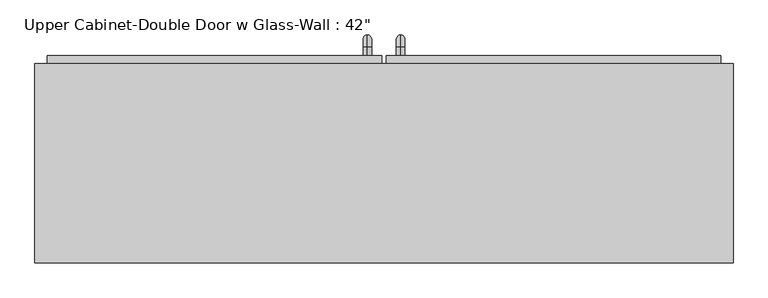
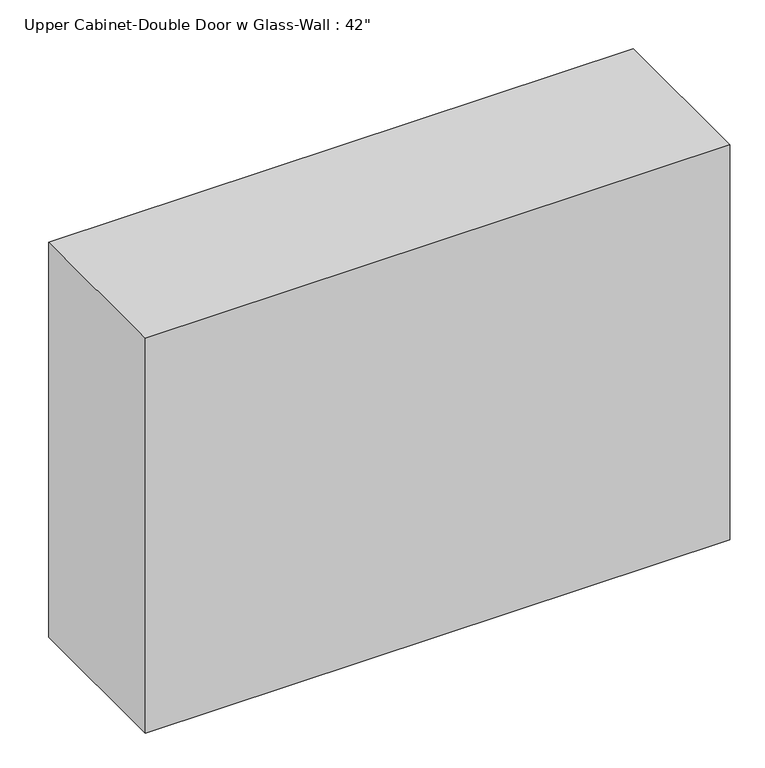
"""IFC4 building model written with IfcOpenShell, lengths in millimetres: furniture geometry."""

from ifc_helpers import new_model, si_unit, point, frame, origin, place, context, project, spatial, polyline, circle_curve, ellipse_curve, trimmed, outline, extrude, faceted_brep, source, transform, mapped, element, save
from ifc_brep_helpers import plane_surface, cylinder_surface, revolved_surface, advanced_brep


def furniture_92d3ea51(model_context):
    return source(origin(), model_context, "Body", "SolidModel", [
        extrude(outline(polyline([(2114.55, 32.9461628), (1390.65, 32.9461628), (1390.65, 544.1211628), (2114.55, 544.1211628), (2114.55, 32.9461628)]), holes=[polyline([(1422.4, 64.6961628), (2082.8, 64.6961628), (2082.8, 512.3711628), (1422.4, 512.3711628), (1422.4, 64.6961628)])]), frame((0.0, 342.9, 0.0), z_axis=(0.0, 1.0, 0.0), x_axis=(0.0, 0.0, 1.0)), (0.0, 0.0, 1.0), 31.75),
        extrude(outline(polyline([(1390.65, -484.5788372), (1390.65, 26.5961628), (2114.55, 26.5961628), (2114.55, -484.5788372), (1390.65, -484.5788372)]), holes=[polyline([(2082.8, -5.1538372), (1422.4, -5.1538372), (1422.4, -452.8288372), (2082.8, -452.8288372), (2082.8, -5.1538372)])]), frame((0.0, 342.9, 0.0), z_axis=(0.0, 1.0, 0.0), x_axis=(0.0, 0.0, 1.0)), (0.0, 0.0, 1.0), 31.75),
        extrude(outline(polyline([(64.6961628, 355.6), (512.3711628, 355.6), (512.3711628, 349.25), (64.6961628, 349.25), (64.6961628, 355.6)])), frame((0.0, 0.0, 1422.4), z_axis=(0.0, 0.0, 1.0), x_axis=(1.0, 0.0, 0.0)), (0.0, 0.0, 1.0), 660.4),
        extrude(outline(polyline([(-452.8288372, 355.6), (-5.1538372, 355.6), (-5.1538372, 349.25), (-452.8288372, 349.25), (-452.8288372, 355.6)])), frame((0.0, 0.0, 1422.4), z_axis=(0.0, 0.0, 1.0), x_axis=(1.0, 0.0, 0.0)), (0.0, 0.0, 1.0), 660.4),
        advanced_brep(
        [(4.3711628, 374.65, 1517.65), (4.3711628, 374.65, 1530.35), (4.3711628, 387.35, 1517.65), (4.3711628, 387.35, 1530.35), (4.3711628, 406.4, 1511.3), (4.3711628, 393.7, 1511.3), (4.3711628, 393.7, 1435.1), (4.3711628, 406.4, 1435.1), (4.3711628, 387.35, 1416.05), (4.3711628, 387.35, 1428.75), (4.3711628, 374.65, 1428.75), (4.3711628, 374.65, 1416.05)],
        [
            (0, 1, circle_curve(frame((4.3711628, 374.65, 1524.0), z_axis=(0.0, -1.0, 0.0), x_axis=(0.0, 0.0, 1.0)), 6.35)),
            (1, 0, circle_curve(frame((4.3711628, 374.65, 1524.0), z_axis=(0.0, -1.0, 0.0), x_axis=(0.0, 0.0, 1.0)), 6.35)),
            (0, 2),
            (2, 3, circle_curve(frame((4.3711628, 387.35, 1524.0), z_axis=(0.0, -1.0, 0.0), x_axis=(0.0, 0.0, 1.0)), 6.35)),
            (3, 1),
            (3, 2, circle_curve(frame((4.3711628, 387.35, 1524.0), z_axis=(0.0, -1.0, 0.0), x_axis=(0.0, 0.0, 1.0)), 6.35)),
            (4, 3, circle_curve(frame((4.3711628, 387.35, 1511.3), z_axis=(1.0, 0.0, 0.0), x_axis=(0.0, 0.0, 1.0)), 19.05)),
            (2, 5, circle_curve(frame((4.3711628, 387.35, 1511.3), z_axis=(-1.0, 0.0, 0.0), x_axis=(0.0, 0.0, 1.0)), 6.35)),
            (5, 4, circle_curve(frame((4.3711628, 400.05, 1511.3), z_axis=(0.0, 0.0, 1.0), x_axis=(0.0, 1.0, 0.0)), 6.35)),
            (4, 5, circle_curve(frame((4.3711628, 400.05, 1511.3), z_axis=(0.0, 0.0, 1.0), x_axis=(0.0, 1.0, 0.0)), 6.35)),
            (5, 6),
            (6, 7, circle_curve(frame((4.3711628, 400.05, 1435.1), z_axis=(0.0, 0.0, 1.0), x_axis=(0.0, 1.0, 0.0)), 6.35)),
            (7, 4),
            (7, 6, circle_curve(frame((4.3711628, 400.05, 1435.1), z_axis=(0.0, 0.0, 1.0), x_axis=(0.0, 1.0, 0.0)), 6.35)),
            (8, 7, circle_curve(frame((4.3711628, 387.35, 1435.1), z_axis=(1.0, 0.0, 0.0), x_axis=(0.0, 1.0, 0.0)), 19.05)),
            (6, 9, circle_curve(frame((4.3711628, 387.35, 1435.1), z_axis=(-1.0, 0.0, 0.0), x_axis=(0.0, 1.0, 0.0)), 6.35)),
            (9, 8, circle_curve(frame((4.3711628, 387.35, 1422.4), z_axis=(0.0, 1.0, 0.0), x_axis=(0.0, 0.0, -1.0)), 6.35)),
            (8, 9, circle_curve(frame((4.3711628, 387.35, 1422.4), z_axis=(0.0, 1.0, 0.0), x_axis=(0.0, 0.0, -1.0)), 6.35)),
            (10, 11, circle_curve(frame((4.3711628, 374.65, 1422.4), z_axis=(0.0, -1.0, 0.0), x_axis=(0.0, 0.0, -1.0)), 6.35)),
            (11, 10, circle_curve(frame((4.3711628, 374.65, 1422.4), z_axis=(0.0, -1.0, 0.0), x_axis=(0.0, 0.0, -1.0)), 6.35)),
            (9, 10),
            (11, 8),
        ],
        [
            plane_surface(frame((-1.9788372, 374.65, 1524.0), z_axis=(0.0, -1.0, 0.0), x_axis=(0.0, 0.0, 1.0))),
            cylinder_surface(frame((4.3711628, 374.65, 1524.0), z_axis=(0.0, -1.0, 0.0), x_axis=(0.0, 0.0, 1.0)), 6.35),
            revolved_surface(trimmed(ellipse_curve(frame((4.3711628, 387.35, 1524.0), z_axis=(0.0, -1.0, 0.0), x_axis=(0.0, 0.0, 1.0)), 6.35, 6.35), [point((4.3711628, 387.35, 1517.65))], [point((4.3711628, 387.35, 1530.35))], True, "CARTESIAN"), (4.3711628, 387.35, 1511.3), (-1.0, 0.0, 0.0)),
            revolved_surface(trimmed(ellipse_curve(frame((4.3711628, 387.35, 1524.0), z_axis=(0.0, -1.0, 0.0), x_axis=(0.0, 0.0, 1.0)), 6.35, 6.35), [point((4.3711628, 387.35, 1530.35))], [point((4.3711628, 387.35, 1517.65))], True, "CARTESIAN"), (4.3711628, 387.35, 1511.3), (-1.0, 0.0, 0.0)),
            cylinder_surface(frame((4.3711628, 400.05, 1511.3), z_axis=(0.0, 0.0, 1.0), x_axis=(0.0, 1.0, 0.0)), 6.35),
            revolved_surface(trimmed(ellipse_curve(frame((4.3711628, 400.05, 1435.1), z_axis=(0.0, 0.0, 1.0), x_axis=(0.0, 1.0, 0.0)), 6.35, 6.35), [point((4.3711628, 393.7, 1435.1))], [point((4.3711628, 406.4, 1435.1))], True, "CARTESIAN"), (4.3711628, 387.35, 1435.1), (-1.0, 0.0, 0.0)),
            revolved_surface(trimmed(ellipse_curve(frame((4.3711628, 400.05, 1435.1), z_axis=(0.0, 0.0, 1.0), x_axis=(0.0, 1.0, 0.0)), 6.35, 6.35), [point((4.3711628, 406.4, 1435.1))], [point((4.3711628, 393.7, 1435.1))], True, "CARTESIAN"), (4.3711628, 387.35, 1435.1), (-1.0, 0.0, 0.0)),
            plane_surface(frame((-1.9788372, 374.65, 1422.4), z_axis=(0.0, -1.0, 0.0), x_axis=(0.0, 0.0, -1.0))),
            cylinder_surface(frame((4.3711628, 387.35, 1422.4), z_axis=(0.0, 1.0, 0.0), x_axis=(0.0, 0.0, -1.0)), 6.35),
        ],
        [
            (0, [[1, 2]]),
            (1, [[-1, 3, 4, 5]]),
            (1, [[-2, -5, 6, -3]]),
            (2, [[7, -4, 8, 9]]),
            (3, [[-8, -6, -7, 10]]),
            (4, [[-9, 11, 12, 13]]),
            (4, [[-10, -13, 14, -11]]),
            (5, [[15, -12, 16, 17]]),
            (6, [[-16, -14, -15, 18]]),
            (7, [[19, 20]]),
            (8, [[-17, 21, -20, 22]]),
            (8, [[-18, -22, -19, -21]]),
        ],
    ),
        advanced_brep(
        [(55.1711628, 374.65, 1517.65), (55.1711628, 374.65, 1530.35), (55.1711628, 387.35, 1517.65), (55.1711628, 387.35, 1530.35), (55.1711628, 406.4, 1511.3), (55.1711628, 393.7, 1511.3), (55.1711628, 393.7, 1435.1), (55.1711628, 406.4, 1435.1), (55.1711628, 387.35, 1416.05), (55.1711628, 387.35, 1428.75), (55.1711628, 374.65, 1428.75), (55.1711628, 374.65, 1416.05)],
        [
            (0, 1, circle_curve(frame((55.1711628, 374.65, 1524.0), z_axis=(0.0, -1.0, 0.0), x_axis=(0.0, 0.0, -1.0)), 6.35)),
            (1, 0, circle_curve(frame((55.1711628, 374.65, 1524.0), z_axis=(0.0, -1.0, 0.0), x_axis=(0.0, 0.0, -1.0)), 6.35)),
            (0, 2),
            (2, 3, circle_curve(frame((55.1711628, 387.35, 1524.0), z_axis=(0.0, -1.0, 0.0), x_axis=(0.0, 0.0, -1.0)), 6.35)),
            (3, 1),
            (3, 2, circle_curve(frame((55.1711628, 387.35, 1524.0), z_axis=(0.0, -1.0, 0.0), x_axis=(0.0, 0.0, -1.0)), 6.35)),
            (4, 3, circle_curve(frame((55.1711628, 387.35, 1511.3), z_axis=(1.0, 0.0, 0.0), x_axis=(0.0, 0.0, 1.0)), 19.05)),
            (2, 5, circle_curve(frame((55.1711628, 387.35, 1511.3), z_axis=(-1.0, 0.0, 0.0), x_axis=(0.0, 0.0, 1.0)), 6.35)),
            (5, 4, circle_curve(frame((55.1711628, 400.05, 1511.3), z_axis=(0.0, 0.0, 1.0), x_axis=(0.0, -1.0, 0.0)), 6.35)),
            (4, 5, circle_curve(frame((55.1711628, 400.05, 1511.3), z_axis=(0.0, 0.0, 1.0), x_axis=(0.0, -1.0, 0.0)), 6.35)),
            (5, 6),
            (6, 7, circle_curve(frame((55.1711628, 400.05, 1435.1), z_axis=(0.0, 0.0, 1.0), x_axis=(0.0, -1.0, 0.0)), 6.35)),
            (7, 4),
            (7, 6, circle_curve(frame((55.1711628, 400.05, 1435.1), z_axis=(0.0, 0.0, 1.0), x_axis=(0.0, -1.0, 0.0)), 6.35)),
            (8, 7, circle_curve(frame((55.1711628, 387.35, 1435.1), z_axis=(1.0, 0.0, 0.0), x_axis=(0.0, 1.0, 0.0)), 19.05)),
            (6, 9, circle_curve(frame((55.1711628, 387.35, 1435.1), z_axis=(-1.0, 0.0, 0.0), x_axis=(0.0, 1.0, 0.0)), 6.35)),
            (9, 8, circle_curve(frame((55.1711628, 387.35, 1422.4), z_axis=(0.0, 1.0, 0.0), x_axis=(0.0, 0.0, 1.0)), 6.35)),
            (8, 9, circle_curve(frame((55.1711628, 387.35, 1422.4), z_axis=(0.0, 1.0, 0.0), x_axis=(0.0, 0.0, 1.0)), 6.35)),
            (10, 11, circle_curve(frame((55.1711628, 374.65, 1422.4), z_axis=(0.0, -1.0, 0.0), x_axis=(0.0, 0.0, 1.0)), 6.35)),
            (11, 10, circle_curve(frame((55.1711628, 374.65, 1422.4), z_axis=(0.0, -1.0, 0.0), x_axis=(0.0, 0.0, 1.0)), 6.35)),
            (9, 10),
            (11, 8),
        ],
        [
            plane_surface(frame((48.8211628, 374.65, 1524.0), z_axis=(0.0, -1.0, 0.0), x_axis=(0.0, 0.0, 1.0))),
            cylinder_surface(frame((55.1711628, 374.65, 1524.0), z_axis=(0.0, -1.0, 0.0), x_axis=(0.0, 0.0, -1.0)), 6.35),
            revolved_surface(trimmed(ellipse_curve(frame((55.1711628, 387.35, 1524.0), z_axis=(0.0, -1.0, 0.0), x_axis=(0.0, 0.0, -1.0)), 6.35, 6.35), [point((55.1711628, 387.35, 1517.65))], [point((55.1711628, 387.35, 1530.35))], True, "CARTESIAN"), (55.1711628, 387.35, 1511.3), (-1.0, 0.0, 0.0)),
            revolved_surface(trimmed(ellipse_curve(frame((55.1711628, 387.35, 1524.0), z_axis=(0.0, -1.0, 0.0), x_axis=(0.0, 0.0, -1.0)), 6.35, 6.35), [point((55.1711628, 387.35, 1530.35))], [point((55.1711628, 387.35, 1517.65))], True, "CARTESIAN"), (55.1711628, 387.35, 1511.3), (-1.0, 0.0, 0.0)),
            cylinder_surface(frame((55.1711628, 400.05, 1511.3), z_axis=(0.0, 0.0, 1.0), x_axis=(0.0, -1.0, 0.0)), 6.35),
            revolved_surface(trimmed(ellipse_curve(frame((55.1711628, 400.05, 1435.1), z_axis=(0.0, 0.0, 1.0), x_axis=(0.0, -1.0, 0.0)), 6.35, 6.35), [point((55.1711628, 393.7, 1435.1))], [point((55.1711628, 406.4, 1435.1))], True, "CARTESIAN"), (55.1711628, 387.35, 1435.1), (-1.0, 0.0, 0.0)),
            revolved_surface(trimmed(ellipse_curve(frame((55.1711628, 400.05, 1435.1), z_axis=(0.0, 0.0, 1.0), x_axis=(0.0, -1.0, 0.0)), 6.35, 6.35), [point((55.1711628, 406.4, 1435.1))], [point((55.1711628, 393.7, 1435.1))], True, "CARTESIAN"), (55.1711628, 387.35, 1435.1), (-1.0, 0.0, 0.0)),
            plane_surface(frame((48.8211628, 374.65, 1422.4), z_axis=(0.0, -1.0, 0.0), x_axis=(0.0, 0.0, -1.0))),
            cylinder_surface(frame((55.1711628, 387.35, 1422.4), z_axis=(0.0, 1.0, 0.0), x_axis=(0.0, 0.0, 1.0)), 6.35),
        ],
        [
            (0, [[1, 2]]),
            (1, [[-1, 3, 4, 5]]),
            (1, [[-2, -5, 6, -3]]),
            (2, [[7, -4, 8, 9]]),
            (3, [[-8, -6, -7, 10]]),
            (4, [[-9, 11, 12, 13]]),
            (4, [[-10, -13, 14, -11]]),
            (5, [[15, -12, 16, 17]]),
            (6, [[-16, -14, -15, 18]]),
            (7, [[19, 20]]),
            (8, [[-17, 21, -20, 22]]),
            (8, [[-18, -22, -19, -21]]),
        ],
    ),
        faceted_brep([(-503.6288372, 57.15, 2133.6), (-503.6288372, 57.15, 1371.6), (563.1711628, 57.15, 1371.6), (563.1711628, 57.15, 2133.6), (-503.6288372, 361.95, 2133.6), (563.1711628, 361.95, 2133.6), (563.1711628, 361.95, 1371.6), (-503.6288372, 361.95, 1371.6), (-484.5788372, 361.95, 2114.55), (-484.5788372, 361.95, 1390.65), (544.1211628, 361.95, 1390.65), (544.1211628, 361.95, 2114.55), (544.1211628, 76.2, 2114.55), (-484.5788372, 76.2, 2114.55), (544.1211628, 76.2, 1390.65), (-484.5788372, 76.2, 1390.65)], [[[0, 1, 2, 3]], [[4, 5, 6, 7], [8, 9, 10, 11]], [[1, 0, 4, 7]], [[2, 1, 7, 6]], [[3, 2, 6, 5]], [[0, 3, 5, 4]], [[8, 11, 12, 13]], [[11, 10, 14, 12]], [[10, 9, 15, 14]], [[9, 8, 13, 15]], [[13, 12, 14, 15]]]),
    ])


if __name__ == "__main__":
    model = new_model("IFC4")
    model_context = context("Model", 3, world=origin())
    ifc_project = project(units=[si_unit("LENGTHUNIT", "METRE", prefix="MILLI")], contexts=[model_context])
    site = spatial("IfcSite", under=ifc_project)
    building = spatial("IfcBuilding", under=site)
    placement = place(None, origin())
    furniture_shape = furniture_92d3ea51(model_context)
    element("IfcFurniture", 1, ObjectType="Upper Cabinet-Double Door w Glass-Wall : 42\"", at=placement, inside=building, context=model_context, shape_type="MappedRepresentation", body=[
        mapped(furniture_shape, transform((0.0, 0.0, 0.0), x_axis=(1.0, 0.0, 0.0), y_axis=(0.0, 1.0, 0.0), z_axis=(0.0, 0.0, 1.0))),
    ])
    save(model, "model.ifc")

# Revit data of these elements
# Type "Upper Cabinet-Double Door w Glass-Wall : 42\""
#   Assembly Code = "C1030410"
#   Depth = 1' - 0"
#   Height = 2' - 6"
#   Top Of Cabinet = 7' - 0"
#   Width = 3' - 6"
#   Cabinet Material = none
#   Door/Drawer Material = none
#   Handle Material = Cabinets - Handles
#   Panel Material = Glass
#   Default Elevation = 0
# Element 1 (IfcFurniture, "Upper Cabinet-Double Door w Glass-Wall : 42\"")
#   Materials on its faces: "Cabinets", "Cabinets - Handles", "Glass"
# Materials
#   "Cabinets - Handles": colour RGB 57 57 57, transparency 0
#   "Glass": class "Glass", colour RGB 0 128 192, transparency 0.75, Description = "Soda Lime Glass", Cost = 0
#   "Cabinets": colour RGB 249 249 249, transparency 0
